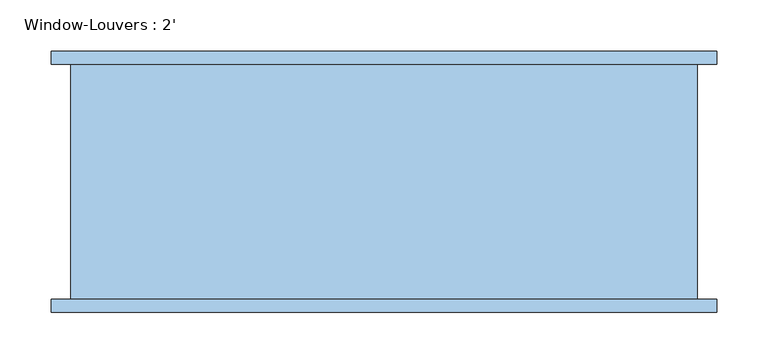
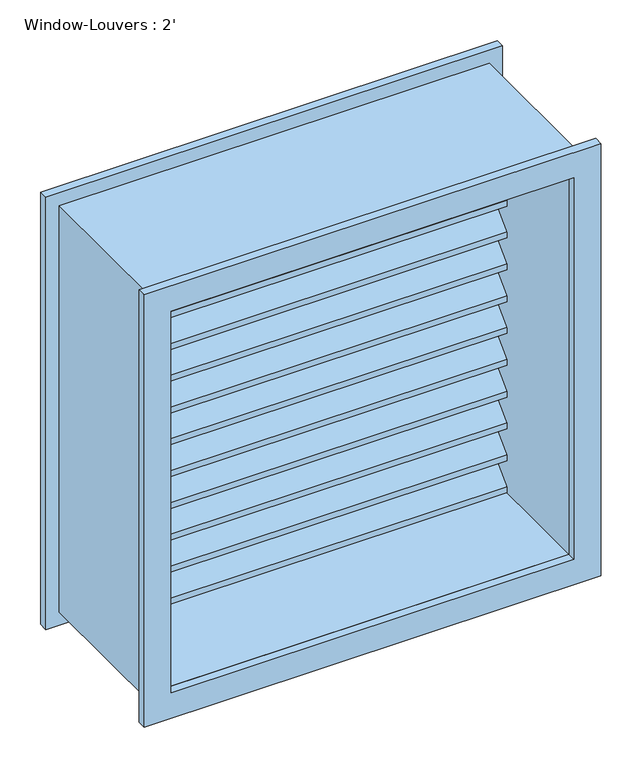
"""IFC4 building model written with IfcOpenShell, lengths in millimetres: window geometry, Window-Louvers : 2'."""

from ifc_helpers import new_model, si_unit, frame, origin, place, context, project, spatial, polyline, outline, extrude, source, transform, mapped, element, save


def window_louvers_2_f2d8fef0(model_context):
    return source(origin(), model_context, "Body", "SweptSolid", [
        extrude(outline(polyline([(107.95, 1419.1754778), (107.95, 1410.1952217), (69.85, 1448.2952217), (31.75, 1410.1952217), (31.75, 1419.1754778), (69.85, 1457.2754778), (107.95, 1419.1754778)])), frame((-285.75, 0.0, 0.0), z_axis=(1.0, 0.0, 0.0), x_axis=(0.0, 1.0, 0.0)), (0.0, 0.0, 1.0), 571.5),
        extrude(outline(polyline([(107.95, 1371.5009557), (107.95, 1362.5206995), (69.85, 1400.6206995), (31.75, 1362.5206995), (31.75, 1371.5009557), (69.85, 1409.6009557), (107.95, 1371.5009557)])), frame((-285.75, 0.0, 0.0), z_axis=(1.0, 0.0, 0.0), x_axis=(0.0, 1.0, 0.0)), (0.0, 0.0, 1.0), 571.5),
        extrude(outline(polyline([(107.95, 1323.8264335), (107.95, 1314.8461774), (69.85, 1352.9461774), (31.75, 1314.8461774), (31.75, 1323.8264335), (69.85, 1361.9264335), (107.95, 1323.8264335)])), frame((-285.75, 0.0, 0.0), z_axis=(1.0, 0.0, 0.0), x_axis=(0.0, 1.0, 0.0)), (0.0, 0.0, 1.0), 571.5),
        extrude(outline(polyline([(107.95, 1276.1519113), (107.95, 1267.1716552), (69.85, 1305.2716552), (31.75, 1267.1716552), (31.75, 1276.1519113), (69.85, 1314.2519113), (107.95, 1276.1519113)])), frame((-285.75, 0.0, 0.0), z_axis=(1.0, 0.0, 0.0), x_axis=(0.0, 1.0, 0.0)), (0.0, 0.0, 1.0), 571.5),
        extrude(outline(polyline([(107.95, 1228.4773891), (107.95, 1219.497133), (69.85, 1257.597133), (31.75, 1219.497133), (31.75, 1228.4773891), (69.85, 1266.5773891), (107.95, 1228.4773891)])), frame((-285.75, 0.0, 0.0), z_axis=(1.0, 0.0, 0.0), x_axis=(0.0, 1.0, 0.0)), (0.0, 0.0, 1.0), 571.5),
        extrude(outline(polyline([(107.95, 1180.802867), (107.95, 1171.8226109), (69.85, 1209.9226109), (31.75, 1171.8226109), (31.75, 1180.802867), (69.85, 1218.902867), (107.95, 1180.802867)])), frame((-285.75, 0.0, 0.0), z_axis=(1.0, 0.0, 0.0), x_axis=(0.0, 1.0, 0.0)), (0.0, 0.0, 1.0), 571.5),
        extrude(outline(polyline([(107.95, 1133.1283448), (107.95, 1124.1480887), (69.85, 1162.2480887), (31.75, 1124.1480887), (31.75, 1133.1283448), (69.85, 1171.2283448), (107.95, 1133.1283448)])), frame((-285.75, 0.0, 0.0), z_axis=(1.0, 0.0, 0.0), x_axis=(0.0, 1.0, 0.0)), (0.0, 0.0, 1.0), 571.5),
        extrude(outline(polyline([(107.95, 1085.4538226), (107.95, 1076.4735665), (69.85, 1114.5735665), (31.75, 1076.4735665), (31.75, 1085.4538226), (69.85, 1123.5538226), (107.95, 1085.4538226)])), frame((-285.75, 0.0, 0.0), z_axis=(1.0, 0.0, 0.0), x_axis=(0.0, 1.0, 0.0)), (0.0, 0.0, 1.0), 571.5),
        extrude(outline(polyline([(107.95, 1037.7793005), (107.95, 1028.7990443), (69.85, 1066.8990443), (31.75, 1028.7990443), (31.75, 1037.7793005), (69.85, 1075.8793005), (107.95, 1037.7793005)])), frame((-285.75, 0.0, 0.0), z_axis=(1.0, 0.0, 0.0), x_axis=(0.0, 1.0, 0.0)), (0.0, 0.0, 1.0), 571.5),
        extrude(outline(polyline([(107.95, 990.1047783), (107.95, 981.1245222), (69.85, 1019.2245222), (31.75, 981.1245222), (31.75, 990.1047783), (69.85, 1028.2047783), (107.95, 990.1047783)])), frame((-285.75, 0.0, 0.0), z_axis=(1.0, 0.0, 0.0), x_axis=(0.0, 1.0, 0.0)), (0.0, 0.0, 1.0), 571.5),
        extrude(outline(polyline([(107.95, 1466.85), (107.95, 1457.8697439), (69.85, 1495.9697439), (31.75, 1457.8697439), (31.75, 1466.85), (69.85, 1504.95), (107.95, 1466.85)])), frame((-285.75, 0.0, 0.0), z_axis=(1.0, 0.0, 0.0), x_axis=(0.0, 1.0, 0.0)), (0.0, 0.0, 1.0), 571.5),
        extrude(outline(polyline([(107.95, 942.4302561), (107.95, 933.45), (69.85, 971.55), (31.75, 933.45), (31.75, 942.4302561), (69.85, 980.5302561), (107.95, 942.4302561)])), frame((-285.75, 0.0, 0.0), z_axis=(1.0, 0.0, 0.0), x_axis=(0.0, 1.0, 0.0)), (0.0, 0.0, 1.0), 571.5),
        extrude(outline(polyline([(1524.0, 304.8), (1524.0, -304.8), (914.4, -304.8), (914.4, 304.8), (1524.0, 304.8)]), holes=[polyline([(1504.95, 285.75), (933.45, 285.75), (933.45, -285.75), (1504.95, -285.75), (1504.95, 285.75)])]), frame((0.0, -120.65, 0.0), z_axis=(0.0, 1.0, 0.0), x_axis=(0.0, 0.0, 1.0)), (0.0, 0.0, 1.0), 228.6),
        extrude(outline(polyline([(1543.05, 323.85), (1543.05, -323.85), (895.35, -323.85), (895.35, 323.85), (1543.05, 323.85)]), holes=[polyline([(1504.95, 285.75), (933.45, 285.75), (933.45, -285.75), (1504.95, -285.75), (1504.95, 285.75)])]), frame((0.0, -133.35, 0.0), z_axis=(0.0, 1.0, 0.0), x_axis=(0.0, 0.0, 1.0)), (0.0, 0.0, 1.0), 12.7),
        extrude(outline(polyline([(1543.05, -323.85), (895.35, -323.85), (895.35, 323.85), (1543.05, 323.85), (1543.05, -323.85)]), holes=[polyline([(1504.95, -285.75), (1504.95, 285.75), (933.45, 285.75), (933.45, -285.75), (1504.95, -285.75)])]), frame((0.0, 107.95, 0.0), z_axis=(0.0, 1.0, 0.0), x_axis=(0.0, 0.0, 1.0)), (0.0, 0.0, 1.0), 12.7),
    ])


if __name__ == "__main__":
    model = new_model("IFC4")
    model_context = context("Model", 3, world=origin())
    ifc_project = project(units=[si_unit("LENGTHUNIT", "METRE", prefix="MILLI")], contexts=[model_context])
    site = spatial("IfcSite", under=ifc_project)
    building = spatial("IfcBuilding", under=site)
    placement = place(None, origin())
    window_louvers_2_shape = window_louvers_2_f2d8fef0(model_context)
    element("IfcWindow", 1, ObjectType="Window-Louvers : 2'", at=placement, inside=building, context=model_context, shape_type="MappedRepresentation", body=[
        mapped(window_louvers_2_shape, transform((0.0, 0.0, 0.0), x_axis=(1.0, 0.0, 0.0), y_axis=(0.0, 1.0, 0.0), z_axis=(0.0, 0.0, 1.0))),
    ])
    save(model, "model.ifc")

# Revit data of these elements
# Type "Window-Louvers : 2'"
#   Type Mark = "25"
#   Assembly Code = "B20"
#   Visual Light Transmittance = 0.9
#   Solar Heat Gain Coefficient = 0.78
#   Max Height = 1' - 11.74264"
#   Height = 2' - 0"
#   Heat Transfer Coefficient (U) = 0.6496 BTU/(h·ft²·°F)
#   Blade Width [instance default] = 1' - 10 1/2"
#   Blade Vertical Thickness = 0' - 0.35355"
#   Blade Thickness = 0' - 0 1/4"
#   Blade Spacing = 0' - 1 1/2"
#   Blade Height = 0' - 1.85355"
#   Blade Depth = 0' - 3"
#   Blade Angle = 45.00°
#   Default Sill Height = 3' - 0"
#   Trim Projection_Exterior = 0' - 0 1/2"
#   Trim Projection_Interior = 0' - 0 1/2"
#   Trim Width_Exterior = 0' - 1 1/2"
#   Trim Width_Interior = 0' - 1 1/2"
#   Width = 2' - 0"
#   Max Blade Count = 12
#   Define Thermal Properties by = 1
#   Blade Count = 12
#   Frame Material = Birch
#   Louver Material = Birch
#   Trim Exterior Material = Birch
#   Trim Interior Material = Birch
#   Thermal Resistance (R) = 0
#   Construction Type Id = ""
#   Wall Closure = (empty or 0)
#   Analytic Construction = (empty or 0)
# Element 1 (IfcWindow, "Window-Louvers : 2'")
#   Materials on its faces: "Birch"
# Materials
#   "Birch": class "Wood", colour RGB 224 178 126, transparency 0, Description = "Betula Alleghaniensis", Cost = 0
